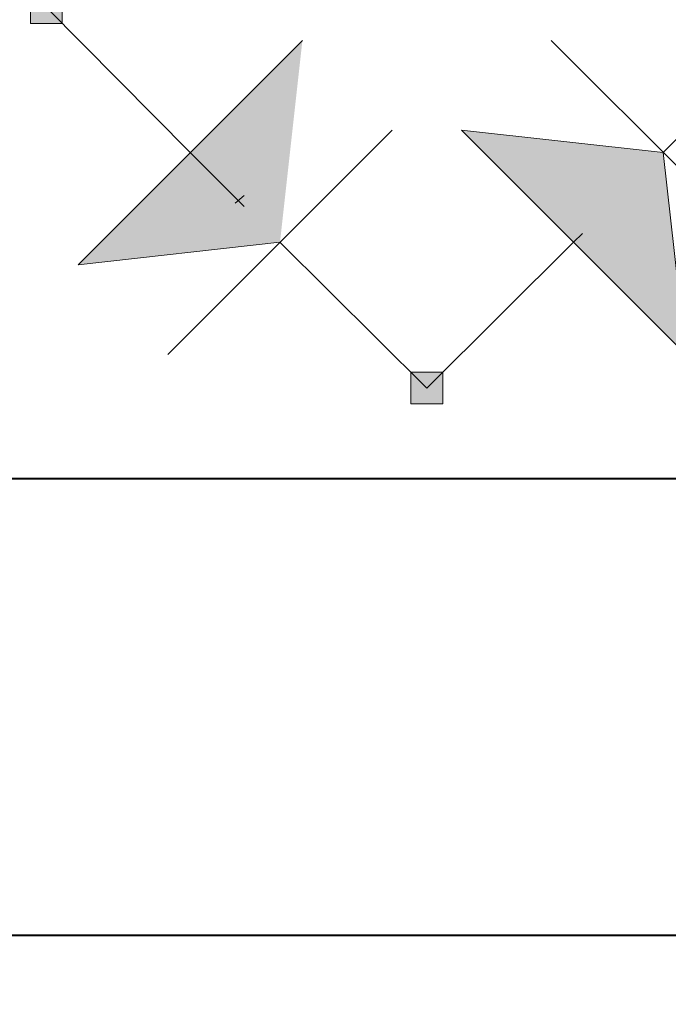
# Model space of a CAD drawing. Units: inches. Extents: x 459864 to 460310, y 324185 to 324787.
# Tile 65 of 112: x 460101.35 to 460114.14, y 324282.12 to 324301.53. Entities that reach past the tile are written whole.
import ezdxf

# ---------------------------------------------------------------- set-up
doc = ezdxf.new("R2010")
doc.units = ezdxf.units.IN
for name, color, linetype, lineweight in [('A-ANNO-DIMS', 2, 'Continuous', 18), ('A-FURN', 8, 'Continuous', 18), ('A-WALL', 7, 'Continuous', 40), ('L-SITE-PATT', 252, 'Continuous', 13)]:
    doc.layers.add(name, color=color, linetype=linetype, lineweight=lineweight)
doc.styles.get("Standard").update_dxf_attribs({"font": 'arial.ttf'})
doc.dimstyles.new('ISO-25', dxfattribs={"dimtxt": 6, "dimasz": 2.5, "dimexe": 1.25, "dimexo": 0.625, "dimtad": 1, "dimdec": 1, "dimlunit": 3, "dimtxsty": 'Standard', "dimcen": 2.5, "dimadec": 0, "dimazin": 0, "dimtfac": 1, "dimtdec": 1, "dimtmove": 0, "dimatfit": 3, "dimfxl": 1, "dimarcsym": 0})

# ---------------------------------------------------------------- blocks, each defined once
blk = doc.blocks.new('Full Wave Bridge')
for p, q in [((0.185922, 0.186729), (0.3, 0.3)), ((0.415786, 0.185084), (0.3, 0.3)), ((0.274311, 0.098341), (0.097534, 0.275118)), ((0.327398, 0.096696), (0.504174, 0.273472)), ((0.504174, 0.273472), (0.486497, 0.114373)), ((0.026823, 0.204407), (0.185922, 0.186729)), ((0.2036, 0.02763), (0.026823, 0.204407)), ((0.398109, 0.025985), (0.574885, 0.202762)), ((0.185922, 0.186729), (0.2036, 0.02763)), ((0.115212, 0.116019), (0.122283, 0.12309)), ((0.115212, 0.116019), (0, 0)), ((0.486497, 0.114373), (0.327398, 0.096696)), ((0.486497, 0.114373), (0.6, 0)), ((0.113504, -0.114373), (0, 0)), ((0.486497, -0.114373), (0.6, 0)), ((0.025116, -0.202762), (0.201892, -0.025985)), ((0.574885, -0.202762), (0.398108, -0.025985)), ((0.095826, -0.273472), (0.272603, -0.096695)), ((0.327398, -0.096695), (0.486497, -0.114373)), ((0.504174, -0.273472), (0.327398, -0.096695)), ((0.113504, -0.114373), (0.120575, -0.121444)), ((0.486497, -0.114373), (0.504174, -0.273472)), ((0.120575, -0.121444), (0.127646, -0.128515)), ((0.127646, -0.128515), (0.134717, -0.135586)), ((0.134717, -0.135586), (0.141788, -0.142657)), ((0.141788, -0.142657), (0.15593, -0.1568)), ((0.155993, -0.148218), (0.148824, -0.154349)), ((0.415786, -0.185084), (0.422857, -0.178013)), ((0.184215, -0.185084), (0.025116, -0.202762)), ((0.184215, -0.185084), (0.3, -0.3)), ((0.415786, -0.185084), (0.3, -0.3))]:
    blk.add_line(p, q)
for points in [[(0.2875, 0.2875), (0.2875, 0.3125), (0.3125, 0.3125), (0.3125, 0.2875)], [(-0.0125, -0.0125), (-0.0125, 0.0125), (0.012501, 0.0125), (0.012501, -0.0125)], [(0.5875, -0.0125), (0.5875, 0.0125), (0.6125, 0.0125), (0.6125, -0.0125)], [(0.2875, -0.3125), (0.2875, -0.2875), (0.3125, -0.2875), (0.3125, -0.3125)]]:
    blk.add_lwpolyline(points, close=True)
for points in [[(0.3125, 0.2875), (0.3125, 0.3125), (0.2875, 0.3125)], [(0.2875, 0.3125), (0.2875, 0.2875), (0.3125, 0.2875)], [(0.327398, 0.096696), (0.486497, 0.114373), (0.504174, 0.273472)], [(0.2036, 0.02763), (0.185922, 0.186729), (0.026823, 0.204407)], [(0.012501, -0.0125), (0.012501, 0.0125), (-0.0125, 0.0125)], [(-0.0125, 0.0125), (-0.0125, -0.0125), (0.012501, -0.0125)], [(0.6125, -0.0125), (0.6125, 0.0125), (0.5875, 0.0125)], [(0.5875, 0.0125), (0.5875, -0.0125), (0.6125, -0.0125)], [(0.025116, -0.202762), (0.184215, -0.185084), (0.201892, -0.025985)], [(0.327398, -0.096695), (0.486497, -0.114373), (0.504174, -0.273472)], [(0.3125, -0.3125), (0.3125, -0.2875), (0.2875, -0.2875)], [(0.2875, -0.2875), (0.2875, -0.3125), (0.3125, -0.3125)]]:
    blk.add_solid(points)
blk = doc.blocks.new('*D73')
at = {"layer": 'A-ANNO-DIMS', "color": 0, "lineweight": -2, "transparency": 16777216}
for p, q in [((460109.617, 324339.904), (460082.316, 324311.465)), ((460063.615, 324291.983), (460080.585, 324309.661))]:
    blk.add_line(p, q, dxfattribs=at)
at = {"layer": 'A-ANNO-DIMS', "color": 0, "transparency": 16777216}
blk.add_solid([(460082.016, 324311.753), (460082.617, 324311.176), (460080.585, 324309.661)], dxfattribs=at)
at = {"layer": 'Defpoints', "color": 0, "transparency": 16777216}
for p in [(460080.585, 324309.661), (460063.615, 324291.983)]:
    blk.add_point(p, dxfattribs=at)
at = {"layer": 'A-ANNO-DIMS', "color": 0, "transparency": 16777216, "insert": (460094.144, 324329.167), "char_height": 6, "attachment_point": 5, "rotation": 46.1701}
blk.add_mtext('R2\'-0 1/2"', dxfattribs=at)

msp = doc.modelspace()

# ---------------------------------------------------------------- hatches: boundary and pattern name
at = {"layer": 'L-SITE-PATT'}
h = msp.add_hatch(dxfattribs=at)
h.set_pattern_fill('DOTS', color=256)
h.paths.add_polyline_path([(460269.804, 324283.483), (460247.115, 324283.483), (460121.929, 324283.483), (460121.929, 324252.473), (460117.429, 324252.473), (460110.124, 324252.473), (460110.124, 324243.287), (460080.83, 324243.287), (460080.83, 324252.473), (460061.115, 324252.473), (460061.115, 324251.882), (460077.909, 324251.882), (460077.909, 324199.483), (460080.83, 324199.483), (460080.83, 324207.553), (460110.124, 324207.553), (460110.124, 324199.483), (460110.813, 324199.483), (460262.115, 324199.483), (460269.804, 324199.483)], flags=17)
edge = h.paths.add_edge_path(flags=0)
edge.add_ellipse((460222.59, 324263.813), major_axis=(-8.485, 8.485), ratio=1, start_angle=405, end_angle=495, ccw=False)
edge.add_line((460214.821, 324254.66), (460214.832, 324254.666))
edge.add_ellipse((460222.59, 324263.813), major_axis=(-8.485, 8.485), ratio=1, start_angle=405, end_angle=495, ccw=False)
edge.add_line((460210.759, 324261.781), (460210.768, 324261.787))
edge.add_ellipse((460222.59, 324263.813), major_axis=(-8.485, 8.485), ratio=1, start_angle=405, end_angle=495, ccw=False)
edge.add_ellipse((460222.59, 324263.813), major_axis=(-8.485, 8.485), ratio=1, start_angle=392.754, end_angle=405, ccw=False)
edge.add_ellipse((460222.59, 324263.813), major_axis=(-8.485, 8.485), ratio=1, start_angle=380.9347, end_angle=392.754, ccw=False)
edge.add_line((460211.337, 324267.985), (460211.34, 324267.985))
edge.add_ellipse((460222.59, 324263.813), major_axis=(-8.485, 8.485), ratio=1, start_angle=380.9347, end_angle=392.754, ccw=False)
edge.add_ellipse((460222.59, 324263.813), major_axis=(-8.485, 8.485), ratio=1, start_angle=347.9015, end_angle=380.9347, ccw=False)
edge.add_ellipse((460222.59, 324263.813), major_axis=(-8.485, 8.485), ratio=1, start_angle=327.0619, end_angle=347.9015, ccw=False)
edge.add_ellipse((460222.59, 324263.813), major_axis=(-8.485, 8.485), ratio=1, start_angle=278.3246, end_angle=327.0619, ccw=False)
edge.add_line((460225.158, 324275.536), (460225.158, 324275.535))
edge.add_ellipse((460222.59, 324263.813), major_axis=(-8.485, 8.485), ratio=1, start_angle=278.3246, end_angle=327.0619, ccw=False)
edge.add_ellipse((460222.59, 324263.813), major_axis=(-8.485, 8.485), ratio=1, start_angle=260.6436, end_angle=278.3246, ccw=False)
edge.add_ellipse((460222.59, 324263.813), major_axis=(-8.485, 8.485), ratio=1, start_angle=225, end_angle=260.6436, ccw=False)
edge.add_line((460234.509, 324265.243), (460234.501, 324265.239))
edge.add_ellipse((460222.59, 324263.813), major_axis=(-8.485, 8.485), ratio=1, start_angle=225, end_angle=260.6436, ccw=False)
edge.add_ellipse((460222.59, 324263.813), major_axis=(-8.485, 8.485), ratio=1, start_angle=495, end_angle=585, ccw=False)
edge.add_line((460234.437, 324261.861), (460234.424, 324261.858))
edge.add_ellipse((460222.59, 324263.813), major_axis=(-8.485, 8.485), ratio=1, start_angle=495, end_angle=585, ccw=False)
edge.add_line((460227.95, 324253.067), (460227.946, 324253.083))
edge.add_ellipse((460222.59, 324263.813), major_axis=(-8.485, 8.485), ratio=1, start_angle=495, end_angle=585, ccw=False)
edge.add_line((460226.223, 324252.369), (460226.211, 324252.38))
edge.add_ellipse((460222.59, 324263.813), major_axis=(-8.485, 8.485), ratio=1, start_angle=495, end_angle=585, ccw=False)
h.paths.add_polyline_path([(460219.651, 324254.347), (460218.461, 324253.545), (460218.275, 324254.789), (460219.642, 324256.542), (460219.625, 324260.848), (460216.11, 324257.333), (460214.35, 324256.978), (460215.416, 324259.356), (460212.524, 324258.496), (460213.137, 324259.93), (460218.507, 324263.813), (460222.59, 324263.813), (460222.59, 324267.807), (460218.176, 324272.212), (460219.026, 324274.639), (460222.59, 324272.811), (460222.59, 324275.423), (460223.057, 324274.825), (460222.675, 324273.492), (460225.912, 324267.135), (460219.625, 324260.848)], flags=0)
edge = h.paths.add_edge_path(flags=0)
edge.add_ellipse((460194.576, 324264.046), major_axis=(-8.485, 8.485), ratio=1, start_angle=495, end_angle=585, ccw=False)
edge.add_line((460199.936, 324253.3), (460199.932, 324253.316))
edge.add_ellipse((460194.576, 324264.046), major_axis=(-8.485, 8.485), ratio=1, start_angle=495, end_angle=585, ccw=False)
edge.add_line((460198.208, 324252.603), (460198.196, 324252.613))
edge.add_ellipse((460194.576, 324264.046), major_axis=(-8.485, 8.485), ratio=1, start_angle=495, end_angle=585, ccw=False)
edge.add_ellipse((460194.576, 324264.046), major_axis=(-8.485, 8.485), ratio=1, start_angle=405, end_angle=495, ccw=False)
edge.add_line((460186.806, 324254.893), (460186.817, 324254.899))
edge.add_ellipse((460194.576, 324264.046), major_axis=(-8.485, 8.485), ratio=1, start_angle=405, end_angle=495, ccw=False)
edge.add_line((460182.744, 324262.014), (460182.753, 324262.02))
edge.add_ellipse((460194.576, 324264.046), major_axis=(-8.485, 8.485), ratio=1, start_angle=405, end_angle=495, ccw=False)
edge.add_ellipse((460194.576, 324264.046), major_axis=(-8.485, 8.485), ratio=1, start_angle=392.754, end_angle=405, ccw=False)
edge.add_ellipse((460194.576, 324264.046), major_axis=(-8.485, 8.485), ratio=1, start_angle=380.9347, end_angle=392.754, ccw=False)
edge.add_line((460183.323, 324268.218), (460183.326, 324268.218))
edge.add_ellipse((460194.576, 324264.046), major_axis=(-8.485, 8.485), ratio=1, start_angle=380.9347, end_angle=392.754, ccw=False)
edge.add_ellipse((460194.576, 324264.046), major_axis=(-8.485, 8.485), ratio=1, start_angle=347.9015, end_angle=380.9347, ccw=False)
edge.add_ellipse((460194.576, 324264.046), major_axis=(-8.485, 8.485), ratio=1, start_angle=327.0619, end_angle=347.9015, ccw=False)
edge.add_ellipse((460194.576, 324264.046), major_axis=(-8.485, 8.485), ratio=1, start_angle=278.3246, end_angle=327.0619, ccw=False)
edge.add_line((460197.144, 324275.769), (460197.143, 324275.768))
edge.add_ellipse((460194.576, 324264.046), major_axis=(-8.485, 8.485), ratio=1, start_angle=278.3246, end_angle=327.0619, ccw=False)
edge.add_ellipse((460194.576, 324264.046), major_axis=(-8.485, 8.485), ratio=1, start_angle=260.6436, end_angle=278.3246, ccw=False)
edge.add_ellipse((460194.576, 324264.046), major_axis=(-8.485, 8.485), ratio=1, start_angle=225, end_angle=260.6436, ccw=False)
edge.add_line((460206.494, 324265.476), (460206.487, 324265.473))
edge.add_ellipse((460194.576, 324264.046), major_axis=(-8.485, 8.485), ratio=1, start_angle=225, end_angle=260.6436, ccw=False)
edge.add_ellipse((460194.576, 324264.046), major_axis=(-8.485, 8.485), ratio=1, start_angle=495, end_angle=585, ccw=False)
edge.add_line((460206.422, 324262.094), (460206.409, 324262.091))
h.paths.add_polyline_path([(460191.61, 324261.081), (460191.637, 324254.58), (460190.447, 324253.778), (460190.261, 324255.023), (460191.628, 324256.775), (460191.61, 324261.081), (460188.096, 324257.566), (460186.335, 324257.211), (460187.402, 324259.589), (460184.509, 324258.729), (460185.123, 324260.163), (460190.493, 324264.046), (460194.576, 324264.046), (460194.576, 324268.04), (460190.161, 324272.446), (460191.011, 324274.872), (460194.576, 324273.044), (460194.576, 324275.657), (460195.043, 324275.058), (460194.661, 324273.725), (460197.897, 324267.368)], flags=0)
edge = h.paths.add_edge_path(flags=0)
edge.add_ellipse((460252.912, 324263.578), major_axis=(-8.485, 8.485), ratio=1, start_angle=405, end_angle=495, ccw=False)
edge.add_line((460241.081, 324261.545), (460241.089, 324261.551))
edge.add_ellipse((460252.912, 324263.578), major_axis=(-8.485, 8.485), ratio=1, start_angle=405, end_angle=495, ccw=False)
edge.add_ellipse((460252.912, 324263.578), major_axis=(-8.485, 8.485), ratio=1, start_angle=392.754, end_angle=405, ccw=False)
edge.add_ellipse((460252.912, 324263.578), major_axis=(-8.485, 8.485), ratio=1, start_angle=380.9347, end_angle=392.754, ccw=False)
edge.add_line((460241.659, 324267.749), (460241.662, 324267.749))
edge.add_ellipse((460252.912, 324263.578), major_axis=(-8.485, 8.485), ratio=1, start_angle=380.9347, end_angle=392.754, ccw=False)
edge.add_ellipse((460252.912, 324263.578), major_axis=(-8.485, 8.485), ratio=1, start_angle=347.9015, end_angle=380.9347, ccw=False)
edge.add_ellipse((460252.912, 324263.578), major_axis=(-8.485, 8.485), ratio=1, start_angle=327.0619, end_angle=347.9015, ccw=False)
edge.add_ellipse((460252.912, 324263.578), major_axis=(-8.485, 8.485), ratio=1, start_angle=278.3246, end_angle=327.0619, ccw=False)
edge.add_line((460255.48, 324275.3), (460255.479, 324275.299))
edge.add_ellipse((460252.912, 324263.578), major_axis=(-8.485, 8.485), ratio=1, start_angle=278.3246, end_angle=327.0619, ccw=False)
edge.add_ellipse((460252.912, 324263.578), major_axis=(-8.485, 8.485), ratio=1, start_angle=260.6436, end_angle=278.3246, ccw=False)
edge.add_ellipse((460252.912, 324263.578), major_axis=(-8.485, 8.485), ratio=1, start_angle=225, end_angle=260.6436, ccw=False)
edge.add_line((460264.83, 324265.007), (460264.823, 324265.004))
edge.add_ellipse((460252.912, 324263.578), major_axis=(-8.485, 8.485), ratio=1, start_angle=225, end_angle=260.6436, ccw=False)
edge.add_ellipse((460252.912, 324263.578), major_axis=(-8.485, 8.485), ratio=1, start_angle=495, end_angle=585, ccw=False)
edge.add_line((460264.758, 324261.626), (460264.745, 324261.622))
edge.add_ellipse((460252.912, 324263.578), major_axis=(-8.485, 8.485), ratio=1, start_angle=495, end_angle=585, ccw=False)
edge.add_line((460258.272, 324252.832), (460258.268, 324252.848))
edge.add_ellipse((460252.912, 324263.578), major_axis=(-8.485, 8.485), ratio=1, start_angle=495, end_angle=585, ccw=False)
edge.add_line((460256.545, 324252.134), (460256.533, 324252.144))
edge.add_ellipse((460252.912, 324263.578), major_axis=(-8.485, 8.485), ratio=1, start_angle=495, end_angle=585, ccw=False)
edge.add_ellipse((460252.912, 324263.578), major_axis=(-8.485, 8.485), ratio=1, start_angle=405, end_angle=495, ccw=False)
edge.add_line((460245.143, 324254.424), (460245.153, 324254.43))
h.paths.add_polyline_path([(460244.672, 324256.742), (460245.738, 324259.12), (460242.846, 324258.26), (460243.459, 324259.694), (460248.829, 324263.578), (460252.912, 324263.578), (460252.912, 324267.571), (460248.497, 324271.977), (460249.348, 324274.403), (460252.912, 324272.576), (460252.912, 324275.188), (460253.379, 324274.589), (460252.997, 324273.257), (460256.233, 324266.899), (460249.946, 324260.612), (460249.973, 324254.111), (460248.783, 324253.309), (460248.597, 324254.554), (460249.964, 324256.306), (460249.946, 324260.612), (460246.432, 324257.097)], flags=0)
edge = h.paths.add_edge_path(flags=0)
edge.add_ellipse((460167.439, 324262.833), major_axis=(-8.485, 8.485), ratio=1, start_angle=495, end_angle=585, ccw=False)
edge.add_line((460172.799, 324252.087), (460172.795, 324252.103))
edge.add_ellipse((460167.439, 324262.833), major_axis=(-8.485, 8.485), ratio=1, start_angle=495, end_angle=585, ccw=False)
edge.add_line((460171.071, 324251.389), (460171.059, 324251.399))
edge.add_ellipse((460167.439, 324262.833), major_axis=(-8.485, 8.485), ratio=1, start_angle=495, end_angle=585, ccw=False)
edge.add_ellipse((460167.439, 324262.833), major_axis=(-8.485, 8.485), ratio=1, start_angle=405, end_angle=495, ccw=False)
edge.add_line((460159.669, 324253.679), (460159.68, 324253.685))
edge.add_ellipse((460167.439, 324262.833), major_axis=(-8.485, 8.485), ratio=1, start_angle=405, end_angle=495, ccw=False)
edge.add_line((460155.607, 324260.8), (460155.616, 324260.806))
edge.add_ellipse((460167.439, 324262.833), major_axis=(-8.485, 8.485), ratio=1, start_angle=405, end_angle=495, ccw=False)
edge.add_ellipse((460167.439, 324262.833), major_axis=(-8.485, 8.485), ratio=1, start_angle=392.754, end_angle=405, ccw=False)
edge.add_ellipse((460167.439, 324262.833), major_axis=(-8.485, 8.485), ratio=1, start_angle=380.9347, end_angle=392.754, ccw=False)
edge.add_line((460156.185, 324267.005), (460156.189, 324267.005))
edge.add_ellipse((460167.439, 324262.833), major_axis=(-8.485, 8.485), ratio=1, start_angle=380.9347, end_angle=392.754, ccw=False)
edge.add_ellipse((460167.439, 324262.833), major_axis=(-8.485, 8.485), ratio=1, start_angle=347.9015, end_angle=380.9347, ccw=False)
edge.add_ellipse((460167.439, 324262.833), major_axis=(-8.485, 8.485), ratio=1, start_angle=327.0619, end_angle=347.9015, ccw=False)
edge.add_ellipse((460167.439, 324262.833), major_axis=(-8.485, 8.485), ratio=1, start_angle=278.3246, end_angle=327.0619, ccw=False)
edge.add_line((460170.007, 324274.556), (460170.006, 324274.554))
edge.add_ellipse((460167.439, 324262.833), major_axis=(-8.485, 8.485), ratio=1, start_angle=278.3246, end_angle=327.0619, ccw=False)
edge.add_ellipse((460167.439, 324262.833), major_axis=(-8.485, 8.485), ratio=1, start_angle=260.6436, end_angle=278.3246, ccw=False)
edge.add_ellipse((460167.439, 324262.833), major_axis=(-8.485, 8.485), ratio=1, start_angle=225, end_angle=260.6436, ccw=False)
edge.add_line((460179.357, 324264.262), (460179.35, 324264.259))
edge.add_ellipse((460167.439, 324262.833), major_axis=(-8.485, 8.485), ratio=1, start_angle=225, end_angle=260.6436, ccw=False)
edge.add_ellipse((460167.439, 324262.833), major_axis=(-8.485, 8.485), ratio=1, start_angle=495, end_angle=585, ccw=False)
edge.add_line((460179.285, 324260.881), (460179.272, 324260.877))
h.paths.add_polyline_path([(460164.473, 324259.867), (460164.5, 324253.366), (460163.31, 324252.565), (460163.124, 324253.809), (460164.491, 324255.561), (460164.473, 324259.867), (460160.958, 324256.353), (460159.198, 324255.998), (460160.265, 324258.375), (460157.372, 324257.515), (460157.986, 324258.949), (460163.356, 324262.833), (460167.439, 324262.833), (460167.439, 324266.826), (460163.024, 324271.232), (460163.874, 324273.659), (460167.439, 324271.831), (460167.439, 324274.443), (460167.905, 324273.844), (460167.524, 324272.512), (460170.76, 324266.154)], flags=0)
edge = h.paths.add_edge_path(flags=0)
edge.add_ellipse((460140.758, 324262.37), major_axis=(-8.485, 8.485), ratio=1, start_angle=495, end_angle=585, ccw=False)
edge.add_line((460146.118, 324251.624), (460146.114, 324251.639))
edge.add_ellipse((460140.758, 324262.37), major_axis=(-8.485, 8.485), ratio=1, start_angle=495, end_angle=585, ccw=False)
edge.add_line((460144.391, 324250.926), (460144.379, 324250.936))
edge.add_ellipse((460140.758, 324262.37), major_axis=(-8.485, 8.485), ratio=1, start_angle=495, end_angle=585, ccw=False)
edge.add_ellipse((460140.758, 324262.37), major_axis=(-8.485, 8.485), ratio=1, start_angle=405, end_angle=495, ccw=False)
edge.add_line((460132.989, 324253.216), (460132.999, 324253.222))
edge.add_ellipse((460140.758, 324262.37), major_axis=(-8.485, 8.485), ratio=1, start_angle=405, end_angle=495, ccw=False)
edge.add_line((460128.927, 324260.337), (460128.935, 324260.343))
edge.add_ellipse((460140.758, 324262.37), major_axis=(-8.485, 8.485), ratio=1, start_angle=405, end_angle=495, ccw=False)
edge.add_ellipse((460140.758, 324262.37), major_axis=(-8.485, 8.485), ratio=1, start_angle=392.754, end_angle=405, ccw=False)
edge.add_ellipse((460140.758, 324262.37), major_axis=(-8.485, 8.485), ratio=1, start_angle=380.9347, end_angle=392.754, ccw=False)
edge.add_line((460129.505, 324266.541), (460129.508, 324266.541))
edge.add_ellipse((460140.758, 324262.37), major_axis=(-8.485, 8.485), ratio=1, start_angle=380.9347, end_angle=392.754, ccw=False)
edge.add_ellipse((460140.758, 324262.37), major_axis=(-8.485, 8.485), ratio=1, start_angle=347.9015, end_angle=380.9347, ccw=False)
edge.add_ellipse((460140.758, 324262.37), major_axis=(-8.485, 8.485), ratio=1, start_angle=327.0619, end_angle=347.9015, ccw=False)
edge.add_ellipse((460140.758, 324262.37), major_axis=(-8.485, 8.485), ratio=1, start_angle=278.3246, end_angle=327.0619, ccw=False)
edge.add_line((460143.326, 324274.092), (460143.325, 324274.091))
edge.add_ellipse((460140.758, 324262.37), major_axis=(-8.485, 8.485), ratio=1, start_angle=278.3246, end_angle=327.0619, ccw=False)
edge.add_ellipse((460140.758, 324262.37), major_axis=(-8.485, 8.485), ratio=1, start_angle=260.6436, end_angle=278.3246, ccw=False)
edge.add_ellipse((460140.758, 324262.37), major_axis=(-8.485, 8.485), ratio=1, start_angle=225, end_angle=260.6436, ccw=False)
edge.add_line((460152.677, 324263.799), (460152.669, 324263.796))
edge.add_ellipse((460140.758, 324262.37), major_axis=(-8.485, 8.485), ratio=1, start_angle=225, end_angle=260.6436, ccw=False)
edge.add_ellipse((460140.758, 324262.37), major_axis=(-8.485, 8.485), ratio=1, start_angle=495, end_angle=585, ccw=False)
edge.add_line((460152.604, 324260.418), (460152.592, 324260.414))
h.paths.add_polyline_path([(460137.792, 324259.404), (460137.819, 324252.903), (460136.629, 324252.101), (460136.443, 324253.346), (460137.81, 324255.098), (460137.792, 324259.404), (460134.278, 324255.889), (460132.518, 324255.534), (460133.584, 324257.912), (460130.692, 324257.052), (460131.305, 324258.486), (460136.675, 324262.37), (460140.758, 324262.37), (460140.758, 324266.363), (460136.343, 324270.769), (460137.194, 324273.195), (460140.758, 324271.367), (460140.758, 324273.98), (460141.225, 324273.381), (460140.843, 324272.049), (460144.079, 324265.691)], flags=0)
h.paths.add_polyline_path([(460110.124, 324227.414), (460080.83, 324227.414), (460080.83, 324235.484), (460110.124, 324235.484)], flags=16)
h.paths.add_polyline_path([(460110.124, 324220.797), (460110.124, 324212.727), (460080.83, 324212.727), (460080.83, 324220.797)], flags=16)
h.paths.add_polyline_path([(460269.804, 324283.483), (460247.115, 324283.483), (460121.929, 324283.483), (460121.929, 324252.473), (460117.429, 324252.473), (460110.124, 324252.473), (460110.124, 324243.287), (460080.83, 324243.287), (460080.83, 324252.473), (460061.115, 324252.473), (460061.115, 324251.882), (460077.909, 324251.882), (460077.909, 324199.483), (460080.83, 324199.483), (460080.83, 324207.553), (460110.124, 324207.553), (460110.124, 324199.483), (460262.115, 324199.483), (460269.804, 324199.483)], flags=17)
h.paths.add_polyline_path([(460219.651, 324254.347), (460218.461, 324253.545), (460218.275, 324254.789), (460219.642, 324256.542), (460219.625, 324260.848), (460216.11, 324257.333), (460214.35, 324256.978), (460215.416, 324259.356), (460212.524, 324258.496), (460213.137, 324259.93), (460218.507, 324263.813), (460222.59, 324263.813), (460220.18, 324266.223), (460215.461, 324265.308), (460211.835, 324266.137), (460216.247, 324267.985), (460218.418, 324267.985), (460222.59, 324263.813), (460222.59, 324267.807), (460218.176, 324272.212), (460219.026, 324274.639), (460222.59, 324272.811), (460222.59, 324275.423), (460223.057, 324274.825), (460222.675, 324273.492), (460225.912, 324267.135), (460222.59, 324263.813), (460231.383, 324263.813), (460228.485, 324262.488), (460224.425, 324261.978), (460228.68, 324257.724), (460228.966, 324254.791), (460227.142, 324256.537), (460227.542, 324254.819), (460227.333, 324253.614), (460222.59, 324259.985), (460222.59, 324255.497), (460221.377, 324256.541), (460220.576, 324261.799), (460219.625, 324260.848)], flags=0)
h.paths.add_polyline_path([(460199.127, 324256.77), (460199.528, 324255.052), (460199.319, 324253.848), (460194.576, 324260.218), (460194.576, 324255.73), (460193.363, 324256.774), (460192.561, 324262.032), (460191.61, 324261.081), (460191.637, 324254.58), (460190.447, 324253.778), (460190.261, 324255.023), (460191.628, 324256.775), (460191.61, 324261.081), (460188.096, 324257.566), (460186.335, 324257.211), (460187.402, 324259.589), (460184.509, 324258.729), (460185.123, 324260.163), (460190.493, 324264.046), (460194.576, 324264.046), (460192.166, 324266.456), (460187.446, 324265.541), (460183.82, 324266.37), (460188.232, 324268.218), (460190.404, 324268.218), (460194.576, 324264.046), (460194.576, 324268.04), (460190.161, 324272.446), (460191.011, 324274.872), (460194.576, 324273.044), (460194.576, 324275.657), (460195.043, 324275.058), (460194.661, 324273.725), (460197.897, 324267.368), (460194.576, 324264.046), (460203.368, 324264.046), (460200.47, 324262.721), (460196.411, 324262.212), (460200.665, 324257.957), (460200.951, 324255.024)], flags=0)
h.paths.add_polyline_path([(460244.672, 324256.742), (460245.738, 324259.12), (460242.846, 324258.26), (460243.459, 324259.694), (460248.829, 324263.578), (460252.912, 324263.578), (460250.502, 324265.987), (460245.783, 324265.072), (460242.156, 324265.901), (460246.568, 324267.749), (460248.74, 324267.749), (460252.912, 324263.578), (460252.912, 324267.571), (460248.497, 324271.977), (460249.348, 324274.403), (460252.912, 324272.576), (460252.912, 324275.188), (460253.379, 324274.589), (460252.997, 324273.257), (460256.233, 324266.899), (460252.912, 324263.578), (460261.705, 324263.578), (460258.806, 324262.252), (460254.747, 324261.743), (460259.002, 324257.488), (460259.288, 324254.555), (460257.463, 324256.301), (460257.864, 324254.583), (460257.655, 324253.379), (460252.912, 324259.749), (460252.912, 324255.261), (460251.699, 324256.305), (460250.897, 324261.563), (460249.946, 324260.612), (460249.973, 324254.111), (460248.783, 324253.309), (460248.597, 324254.554), (460249.964, 324256.306), (460249.946, 324260.612), (460246.432, 324257.097)], flags=0)
h.paths.add_polyline_path([(460173.528, 324256.743), (460173.814, 324253.811), (460171.99, 324255.556), (460172.39, 324253.838), (460172.182, 324252.634), (460167.439, 324259.004), (460167.439, 324254.516), (460166.226, 324255.56), (460165.424, 324260.818), (460164.473, 324259.867), (460164.5, 324253.366), (460163.31, 324252.565), (460163.124, 324253.809), (460164.491, 324255.561), (460164.473, 324259.867), (460160.958, 324256.353), (460159.198, 324255.998), (460160.265, 324258.375), (460157.372, 324257.515), (460157.986, 324258.949), (460163.356, 324262.833), (460167.439, 324262.833), (460165.029, 324265.243), (460160.309, 324264.327), (460156.683, 324265.156), (460161.095, 324267.005), (460163.267, 324267.005), (460167.439, 324262.833), (460167.439, 324266.826), (460163.024, 324271.232), (460163.874, 324273.659), (460167.439, 324271.831), (460167.439, 324274.443), (460167.905, 324273.844), (460167.524, 324272.512), (460170.76, 324266.154), (460167.439, 324262.833), (460176.231, 324262.833), (460173.333, 324261.507), (460169.274, 324260.998)], flags=0)
h.paths.add_polyline_path([(460146.848, 324256.28), (460147.134, 324253.347), (460145.31, 324255.093), (460145.71, 324253.375), (460145.501, 324252.171), (460140.758, 324258.541), (460140.758, 324254.053), (460139.545, 324255.097), (460138.744, 324260.355), (460137.792, 324259.404), (460137.819, 324252.903), (460136.629, 324252.101), (460136.443, 324253.346), (460137.81, 324255.098), (460137.792, 324259.404), (460134.278, 324255.889), (460132.518, 324255.534), (460133.584, 324257.912), (460130.692, 324257.052), (460131.305, 324258.486), (460136.675, 324262.37), (460140.758, 324262.37), (460138.348, 324264.779), (460133.629, 324263.864), (460130.002, 324264.693), (460134.414, 324266.541), (460136.586, 324266.541), (460140.758, 324262.37), (460140.758, 324266.363), (460136.343, 324270.769), (460137.194, 324273.195), (460140.758, 324271.367), (460140.758, 324273.98), (460141.225, 324273.381), (460140.843, 324272.049), (460144.079, 324265.691), (460140.758, 324262.37), (460149.551, 324262.37), (460146.653, 324261.044), (460142.593, 324260.535)], flags=0)
edge = h.paths.add_edge_path()
edge.add_line((460269.804, 324272.549), (460260.881, 324272.549))
edge.add_ellipse((460252.912, 324263.578), major_axis=(-8.485, 8.485), ratio=1, start_angle=260.6436, end_angle=273.3846, ccw=False)
edge.add_line((460262.283, 324271.092), (460262.261, 324271.091))
edge.add_ellipse((460252.912, 324263.578), major_axis=(-8.485, 8.485), ratio=1, start_angle=260.6436, end_angle=273.3846, ccw=False)
edge.add_ellipse((460252.912, 324263.578), major_axis=(-8.485, 8.485), ratio=1, start_angle=225, end_angle=260.6436, ccw=False)
edge.add_line((460263.609, 324269.063), (460263.572, 324269.058))
edge.add_ellipse((460252.912, 324263.578), major_axis=(-8.485, 8.485), ratio=1, start_angle=225, end_angle=260.6436, ccw=False)
edge.add_line((460264.615, 324266.306), (460264.585, 324266.305))
edge.add_ellipse((460252.912, 324263.578), major_axis=(-8.485, 8.485), ratio=1, start_angle=225, end_angle=260.6436, ccw=False)
edge.add_line((460264.83, 324265.007), (460264.823, 324265.004))
edge.add_ellipse((460252.912, 324263.578), major_axis=(-8.485, 8.485), ratio=1, start_angle=225, end_angle=260.6436, ccw=False)
edge.add_ellipse((460252.912, 324263.578), major_axis=(-8.485, 8.485), ratio=1, start_angle=495, end_angle=585, ccw=False)
edge.add_line((460264.758, 324261.626), (460264.745, 324261.622))
edge.add_ellipse((460252.912, 324263.578), major_axis=(-8.485, 8.485), ratio=1, start_angle=495, end_angle=585, ccw=False)
edge.add_line((460263.442, 324257.739), (460263.389, 324257.779))
edge.add_ellipse((460252.912, 324263.578), major_axis=(-8.485, 8.485), ratio=1, start_angle=495, end_angle=585, ccw=False)
edge.add_line((460258.128, 324252.744), (460258.102, 324252.779))
edge.add_ellipse((460252.912, 324263.578), major_axis=(-8.485, 8.485), ratio=1, start_angle=495, end_angle=585, ccw=False)
edge.add_line((460256.545, 324252.134), (460256.533, 324252.144))
edge.add_ellipse((460252.912, 324263.578), major_axis=(-8.485, 8.485), ratio=1, start_angle=495, end_angle=585, ccw=False)
edge.add_ellipse((460252.912, 324263.578), major_axis=(-8.485, 8.485), ratio=1, start_angle=405, end_angle=495, ccw=False)
edge.add_line((460250.594, 324251.78), (460250.605, 324251.82))
edge.add_ellipse((460252.912, 324263.578), major_axis=(-8.485, 8.485), ratio=1, start_angle=405, end_angle=495, ccw=False)
edge.add_line((460245.143, 324254.424), (460245.153, 324254.43))
edge.add_ellipse((460252.912, 324263.578), major_axis=(-8.485, 8.485), ratio=1, start_angle=405, end_angle=495, ccw=False)
edge.add_line((460243.525, 324256.059), (460243.56, 324256.091))
edge.add_ellipse((460252.912, 324263.578), major_axis=(-8.485, 8.485), ratio=1, start_angle=405, end_angle=495, ccw=False)
edge.add_line((460241.44, 324259.893), (460241.522, 324259.896))
edge.add_ellipse((460252.912, 324263.578), major_axis=(-8.485, 8.485), ratio=1, start_angle=405, end_angle=495, ccw=False)
edge.add_line((460241.081, 324261.545), (460241.089, 324261.551))
edge.add_ellipse((460252.912, 324263.578), major_axis=(-8.485, 8.485), ratio=1, start_angle=405, end_angle=495, ccw=False)
edge.add_ellipse((460252.912, 324263.578), major_axis=(-8.485, 8.485), ratio=1, start_angle=392.754, end_angle=405, ccw=False)
edge.add_line((460241.05, 324265.438), (460241.063, 324265.443))
edge.add_ellipse((460252.912, 324263.578), major_axis=(-8.485, 8.485), ratio=1, start_angle=392.754, end_angle=405, ccw=False)
edge.add_ellipse((460252.912, 324263.578), major_axis=(-8.485, 8.485), ratio=1, start_angle=380.9347, end_angle=392.754, ccw=False)
edge.add_line((460241.452, 324267.176), (460241.469, 324267.171))
edge.add_ellipse((460252.912, 324263.578), major_axis=(-8.485, 8.485), ratio=1, start_angle=380.9347, end_angle=392.754, ccw=False)
edge.add_line((460241.659, 324267.749), (460241.662, 324267.749))
edge.add_ellipse((460252.912, 324263.578), major_axis=(-8.485, 8.485), ratio=1, start_angle=380.9347, end_angle=392.754, ccw=False)
edge.add_ellipse((460252.912, 324263.578), major_axis=(-8.485, 8.485), ratio=1, start_angle=356.6154, end_angle=380.9347, ccw=False)
edge.add_line((460244.88, 324272.488), (460244.713, 324272.549))
edge.add_line((460244.713, 324272.549), (460230.817, 324272.549))
edge.add_ellipse((460222.59, 324263.813), major_axis=(-8.485, 8.485), ratio=1, start_angle=260.6436, end_angle=271.7178, ccw=False)
edge.add_ellipse((460222.59, 324263.813), major_axis=(-8.485, 8.485), ratio=1, start_angle=225, end_angle=260.6436, ccw=False)
edge.add_line((460233.287, 324269.299), (460233.25, 324269.294))
edge.add_ellipse((460222.59, 324263.813), major_axis=(-8.485, 8.485), ratio=1, start_angle=225, end_angle=260.6436, ccw=False)
edge.add_line((460234.294, 324266.541), (460234.264, 324266.541))
edge.add_ellipse((460222.59, 324263.813), major_axis=(-8.485, 8.485), ratio=1, start_angle=225, end_angle=260.6436, ccw=False)
edge.add_line((460234.509, 324265.243), (460234.501, 324265.239))
edge.add_ellipse((460222.59, 324263.813), major_axis=(-8.485, 8.485), ratio=1, start_angle=225, end_angle=260.6436, ccw=False)
edge.add_ellipse((460222.59, 324263.813), major_axis=(-8.485, 8.485), ratio=1, start_angle=495, end_angle=585, ccw=False)
edge.add_line((460234.437, 324261.861), (460234.424, 324261.858))
edge.add_ellipse((460222.59, 324263.813), major_axis=(-8.485, 8.485), ratio=1, start_angle=495, end_angle=585, ccw=False)
edge.add_line((460233.121, 324257.975), (460233.068, 324258.015))
edge.add_ellipse((460222.59, 324263.813), major_axis=(-8.485, 8.485), ratio=1, start_angle=495, end_angle=585, ccw=False)
edge.add_line((460227.806, 324252.979), (460227.78, 324253.014))
edge.add_ellipse((460222.59, 324263.813), major_axis=(-8.485, 8.485), ratio=1, start_angle=495, end_angle=585, ccw=False)
edge.add_line((460226.223, 324252.369), (460226.211, 324252.38))
edge.add_ellipse((460222.59, 324263.813), major_axis=(-8.485, 8.485), ratio=1, start_angle=495, end_angle=585, ccw=False)
edge.add_ellipse((460222.59, 324263.813), major_axis=(-8.485, 8.485), ratio=1, start_angle=405, end_angle=495, ccw=False)
edge.add_line((460220.272, 324252.016), (460220.283, 324252.055))
edge.add_ellipse((460222.59, 324263.813), major_axis=(-8.485, 8.485), ratio=1, start_angle=405, end_angle=495, ccw=False)
edge.add_line((460214.821, 324254.66), (460214.832, 324254.666))
edge.add_ellipse((460222.59, 324263.813), major_axis=(-8.485, 8.485), ratio=1, start_angle=405, end_angle=495, ccw=False)
edge.add_line((460213.203, 324256.295), (460213.239, 324256.327))
edge.add_ellipse((460222.59, 324263.813), major_axis=(-8.485, 8.485), ratio=1, start_angle=405, end_angle=495, ccw=False)
edge.add_line((460211.118, 324260.128), (460211.201, 324260.131))
edge.add_ellipse((460222.59, 324263.813), major_axis=(-8.485, 8.485), ratio=1, start_angle=405, end_angle=495, ccw=False)
edge.add_line((460210.759, 324261.781), (460210.768, 324261.787))
edge.add_ellipse((460222.59, 324263.813), major_axis=(-8.485, 8.485), ratio=1, start_angle=405, end_angle=495, ccw=False)
edge.add_ellipse((460222.59, 324263.813), major_axis=(-8.485, 8.485), ratio=1, start_angle=392.754, end_angle=405, ccw=False)
edge.add_line((460210.729, 324265.673), (460210.741, 324265.678))
edge.add_ellipse((460222.59, 324263.813), major_axis=(-8.485, 8.485), ratio=1, start_angle=392.754, end_angle=405, ccw=False)
edge.add_ellipse((460222.59, 324263.813), major_axis=(-8.485, 8.485), ratio=1, start_angle=380.9347, end_angle=392.754, ccw=False)
edge.add_line((460211.13, 324267.412), (460211.147, 324267.407))
edge.add_ellipse((460222.59, 324263.813), major_axis=(-8.485, 8.485), ratio=1, start_angle=380.9347, end_angle=392.754, ccw=False)
edge.add_line((460211.337, 324267.985), (460211.34, 324267.985))
edge.add_ellipse((460222.59, 324263.813), major_axis=(-8.485, 8.485), ratio=1, start_angle=380.9347, end_angle=392.754, ccw=False)
edge.add_ellipse((460222.59, 324263.813), major_axis=(-8.485, 8.485), ratio=1, start_angle=358.2822, end_angle=380.9347, ccw=False)
edge.add_line((460213.705, 324271.902), (460213.709, 324271.869))
edge.add_ellipse((460222.59, 324263.813), major_axis=(-8.485, 8.485), ratio=1, start_angle=358.2822, end_angle=380.9347, ccw=False)
edge.add_line((460214.363, 324272.549), (460203.078, 324272.549))
edge.add_line((460203.078, 324272.549), (460203.06, 324272.531))
edge.add_ellipse((460194.576, 324264.046), major_axis=(-8.485, 8.485), ratio=1, start_angle=260.6436, end_angle=270.1168, ccw=False)
edge.add_line((460203.957, 324271.561), (460203.921, 324271.56))
edge.add_ellipse((460194.576, 324264.046), major_axis=(-8.485, 8.485), ratio=1, start_angle=260.6436, end_angle=270.1168, ccw=False)
edge.add_ellipse((460194.576, 324264.046), major_axis=(-8.485, 8.485), ratio=1, start_angle=225, end_angle=260.6436, ccw=False)
edge.add_line((460205.272, 324269.532), (460205.235, 324269.527))
edge.add_ellipse((460194.576, 324264.046), major_axis=(-8.485, 8.485), ratio=1, start_angle=225, end_angle=260.6436, ccw=False)
edge.add_line((460206.279, 324266.774), (460206.249, 324266.774))
edge.add_ellipse((460194.576, 324264.046), major_axis=(-8.485, 8.485), ratio=1, start_angle=225, end_angle=260.6436, ccw=False)
edge.add_line((460206.494, 324265.476), (460206.487, 324265.473))
edge.add_ellipse((460194.576, 324264.046), major_axis=(-8.485, 8.485), ratio=1, start_angle=225, end_angle=260.6436, ccw=False)
edge.add_ellipse((460194.576, 324264.046), major_axis=(-8.485, 8.485), ratio=1, start_angle=495, end_angle=585, ccw=False)
edge.add_line((460206.422, 324262.094), (460206.409, 324262.091))
edge.add_ellipse((460194.576, 324264.046), major_axis=(-8.485, 8.485), ratio=1, start_angle=495, end_angle=585, ccw=False)
edge.add_line((460205.106, 324258.208), (460205.053, 324258.248))
edge.add_ellipse((460194.576, 324264.046), major_axis=(-8.485, 8.485), ratio=1, start_angle=495, end_angle=585, ccw=False)
edge.add_line((460199.792, 324253.212), (460199.766, 324253.248))
edge.add_ellipse((460194.576, 324264.046), major_axis=(-8.485, 8.485), ratio=1, start_angle=495, end_angle=585, ccw=False)
edge.add_line((460198.208, 324252.603), (460198.196, 324252.613))
edge.add_ellipse((460194.576, 324264.046), major_axis=(-8.485, 8.485), ratio=1, start_angle=495, end_angle=585, ccw=False)
edge.add_ellipse((460194.576, 324264.046), major_axis=(-8.485, 8.485), ratio=1, start_angle=405, end_angle=495, ccw=False)
edge.add_line((460192.258, 324252.249), (460192.268, 324252.289))
edge.add_ellipse((460194.576, 324264.046), major_axis=(-8.485, 8.485), ratio=1, start_angle=405, end_angle=495, ccw=False)
edge.add_line((460186.806, 324254.893), (460186.817, 324254.899))
edge.add_ellipse((460194.576, 324264.046), major_axis=(-8.485, 8.485), ratio=1, start_angle=405, end_angle=495, ccw=False)
edge.add_line((460185.188, 324256.528), (460185.224, 324256.56))
edge.add_ellipse((460194.576, 324264.046), major_axis=(-8.485, 8.485), ratio=1, start_angle=405, end_angle=495, ccw=False)
edge.add_line((460183.104, 324260.362), (460183.186, 324260.365))
edge.add_ellipse((460194.576, 324264.046), major_axis=(-8.485, 8.485), ratio=1, start_angle=405, end_angle=495, ccw=False)
edge.add_line((460182.744, 324262.014), (460182.753, 324262.02))
edge.add_ellipse((460194.576, 324264.046), major_axis=(-8.485, 8.485), ratio=1, start_angle=405, end_angle=495, ccw=False)
edge.add_ellipse((460194.576, 324264.046), major_axis=(-8.485, 8.485), ratio=1, start_angle=392.754, end_angle=405, ccw=False)
edge.add_line((460182.714, 324265.906), (460182.726, 324265.912))
edge.add_ellipse((460194.576, 324264.046), major_axis=(-8.485, 8.485), ratio=1, start_angle=392.754, end_angle=405, ccw=False)
edge.add_ellipse((460194.576, 324264.046), major_axis=(-8.485, 8.485), ratio=1, start_angle=380.9347, end_angle=392.754, ccw=False)
edge.add_line((460183.116, 324267.645), (460183.133, 324267.64))
edge.add_ellipse((460194.576, 324264.046), major_axis=(-8.485, 8.485), ratio=1, start_angle=380.9347, end_angle=392.754, ccw=False)
edge.add_line((460183.323, 324268.218), (460183.326, 324268.218))
edge.add_ellipse((460194.576, 324264.046), major_axis=(-8.485, 8.485), ratio=1, start_angle=380.9347, end_angle=392.754, ccw=False)
edge.add_ellipse((460194.576, 324264.046), major_axis=(-8.485, 8.485), ratio=1, start_angle=359.8832, end_angle=380.9347, ccw=False)
edge.add_line((460184.491, 324270.611), (460184.553, 324270.611))
edge.add_ellipse((460194.576, 324264.046), major_axis=(-8.485, 8.485), ratio=1, start_angle=359.8832, end_angle=380.9347, ccw=False)
edge.add_line((460185.346, 324271.76), (460185.379, 324271.728))
edge.add_ellipse((460194.576, 324264.046), major_axis=(-8.485, 8.485), ratio=1, start_angle=359.8832, end_angle=380.9347, ccw=False)
edge.add_line((460185.697, 324272.086), (460185.633, 324272.549))
edge.add_line((460185.633, 324272.549), (460174.683, 324272.549))
edge.add_line((460174.683, 324272.549), (460174.606, 324272.457))
edge.add_ellipse((460167.439, 324262.833), major_axis=(-8.485, 8.485), ratio=1, start_angle=260.6436, end_angle=278.3246, ccw=False)
edge.add_ellipse((460167.439, 324262.833), major_axis=(-8.485, 8.485), ratio=1, start_angle=225, end_angle=260.6436, ccw=False)
edge.add_line((460178.135, 324268.318), (460178.098, 324268.313))
edge.add_ellipse((460167.439, 324262.833), major_axis=(-8.485, 8.485), ratio=1, start_angle=225, end_angle=260.6436, ccw=False)
edge.add_line((460179.142, 324265.561), (460179.112, 324265.56))
edge.add_ellipse((460167.439, 324262.833), major_axis=(-8.485, 8.485), ratio=1, start_angle=225, end_angle=260.6436, ccw=False)
edge.add_line((460179.357, 324264.262), (460179.35, 324264.259))
edge.add_ellipse((460167.439, 324262.833), major_axis=(-8.485, 8.485), ratio=1, start_angle=225, end_angle=260.6436, ccw=False)
edge.add_ellipse((460167.439, 324262.833), major_axis=(-8.485, 8.485), ratio=1, start_angle=495, end_angle=585, ccw=False)
edge.add_line((460179.285, 324260.881), (460179.272, 324260.877))
edge.add_ellipse((460167.439, 324262.833), major_axis=(-8.485, 8.485), ratio=1, start_angle=495, end_angle=585, ccw=False)
edge.add_line((460177.969, 324256.994), (460177.916, 324257.034))
edge.add_ellipse((460167.439, 324262.833), major_axis=(-8.485, 8.485), ratio=1, start_angle=495, end_angle=585, ccw=False)
edge.add_line((460172.655, 324251.999), (460172.629, 324252.034))
edge.add_ellipse((460167.439, 324262.833), major_axis=(-8.485, 8.485), ratio=1, start_angle=495, end_angle=585, ccw=False)
edge.add_line((460171.071, 324251.389), (460171.059, 324251.399))
edge.add_ellipse((460167.439, 324262.833), major_axis=(-8.485, 8.485), ratio=1, start_angle=495, end_angle=585, ccw=False)
edge.add_ellipse((460167.439, 324262.833), major_axis=(-8.485, 8.485), ratio=1, start_angle=405, end_angle=495, ccw=False)
edge.add_line((460165.121, 324251.036), (460165.131, 324251.075))
edge.add_ellipse((460167.439, 324262.833), major_axis=(-8.485, 8.485), ratio=1, start_angle=405, end_angle=495, ccw=False)
edge.add_line((460159.669, 324253.679), (460159.68, 324253.685))
edge.add_ellipse((460167.439, 324262.833), major_axis=(-8.485, 8.485), ratio=1, start_angle=405, end_angle=495, ccw=False)
edge.add_line((460158.051, 324255.314), (460158.087, 324255.347))
edge.add_ellipse((460167.439, 324262.833), major_axis=(-8.485, 8.485), ratio=1, start_angle=405, end_angle=495, ccw=False)
edge.add_line((460155.967, 324259.148), (460156.049, 324259.151))
edge.add_ellipse((460167.439, 324262.833), major_axis=(-8.485, 8.485), ratio=1, start_angle=405, end_angle=495, ccw=False)
edge.add_line((460155.607, 324260.8), (460155.616, 324260.806))
edge.add_ellipse((460167.439, 324262.833), major_axis=(-8.485, 8.485), ratio=1, start_angle=405, end_angle=495, ccw=False)
edge.add_ellipse((460167.439, 324262.833), major_axis=(-8.485, 8.485), ratio=1, start_angle=392.754, end_angle=405, ccw=False)
edge.add_line((460155.577, 324264.693), (460155.589, 324264.698))
edge.add_ellipse((460167.439, 324262.833), major_axis=(-8.485, 8.485), ratio=1, start_angle=392.754, end_angle=405, ccw=False)
edge.add_ellipse((460167.439, 324262.833), major_axis=(-8.485, 8.485), ratio=1, start_angle=380.9347, end_angle=392.754, ccw=False)
edge.add_line((460155.979, 324266.432), (460155.996, 324266.426))
edge.add_ellipse((460167.439, 324262.833), major_axis=(-8.485, 8.485), ratio=1, start_angle=380.9347, end_angle=392.754, ccw=False)
edge.add_line((460156.185, 324267.005), (460156.189, 324267.005))
edge.add_ellipse((460167.439, 324262.833), major_axis=(-8.485, 8.485), ratio=1, start_angle=380.9347, end_angle=392.754, ccw=False)
edge.add_ellipse((460167.439, 324262.833), major_axis=(-8.485, 8.485), ratio=1, start_angle=350.9345, end_angle=380.9347, ccw=False)
edge.add_line((460157.363, 324269.397), (460157.414, 324269.397))
edge.add_ellipse((460167.439, 324262.833), major_axis=(-8.485, 8.485), ratio=1, start_angle=350.9345, end_angle=380.9347, ccw=False)
edge.add_line((460158.221, 324270.535), (460158.236, 324270.519))
edge.add_ellipse((460167.439, 324262.833), major_axis=(-8.485, 8.485), ratio=1, start_angle=350.9345, end_angle=380.9347, ccw=False)
edge.add_line((460159.379, 324271.753), (460159.419, 324271.738))
edge.add_ellipse((460167.439, 324262.833), major_axis=(-8.485, 8.485), ratio=1, start_angle=350.9345, end_angle=380.9347, ccw=False)
edge.add_line((460160.396, 324272.549), (460147.112, 324272.549))
edge.add_ellipse((460140.758, 324262.37), major_axis=(-8.485, 8.485), ratio=1, start_angle=278.3246, end_angle=283.0261, ccw=False)
edge.add_ellipse((460140.758, 324262.37), major_axis=(-8.485, 8.485), ratio=1, start_angle=260.6436, end_angle=278.3246, ccw=False)
edge.add_ellipse((460140.758, 324262.37), major_axis=(-8.485, 8.485), ratio=1, start_angle=225, end_angle=260.6436, ccw=False)
edge.add_line((460151.455, 324267.855), (460151.418, 324267.85))
edge.add_ellipse((460140.758, 324262.37), major_axis=(-8.485, 8.485), ratio=1, start_angle=225, end_angle=260.6436, ccw=False)
edge.add_line((460152.462, 324265.098), (460152.431, 324265.097))
edge.add_ellipse((460140.758, 324262.37), major_axis=(-8.485, 8.485), ratio=1, start_angle=225, end_angle=260.6436, ccw=False)
edge.add_line((460152.677, 324263.799), (460152.669, 324263.796))
edge.add_ellipse((460140.758, 324262.37), major_axis=(-8.485, 8.485), ratio=1, start_angle=225, end_angle=260.6436, ccw=False)
edge.add_ellipse((460140.758, 324262.37), major_axis=(-8.485, 8.485), ratio=1, start_angle=495, end_angle=585, ccw=False)
edge.add_line((460152.604, 324260.418), (460152.592, 324260.414))
edge.add_ellipse((460140.758, 324262.37), major_axis=(-8.485, 8.485), ratio=1, start_angle=495, end_angle=585, ccw=False)
edge.add_line((460151.288, 324256.531), (460151.235, 324256.571))
edge.add_ellipse((460140.758, 324262.37), major_axis=(-8.485, 8.485), ratio=1, start_angle=495, end_angle=585, ccw=False)
edge.add_line((460145.974, 324251.535), (460145.948, 324251.571))
edge.add_ellipse((460140.758, 324262.37), major_axis=(-8.485, 8.485), ratio=1, start_angle=495, end_angle=585, ccw=False)
edge.add_line((460144.391, 324250.926), (460144.379, 324250.936))
edge.add_ellipse((460140.758, 324262.37), major_axis=(-8.485, 8.485), ratio=1, start_angle=495, end_angle=585, ccw=False)
edge.add_ellipse((460140.758, 324262.37), major_axis=(-8.485, 8.485), ratio=1, start_angle=405, end_angle=495, ccw=False)
edge.add_line((460138.44, 324250.572), (460138.451, 324250.612))
edge.add_ellipse((460140.758, 324262.37), major_axis=(-8.485, 8.485), ratio=1, start_angle=405, end_angle=495, ccw=False)
edge.add_line((460132.989, 324253.216), (460132.999, 324253.222))
edge.add_ellipse((460140.758, 324262.37), major_axis=(-8.485, 8.485), ratio=1, start_angle=405, end_angle=495, ccw=False)
edge.add_line((460131.371, 324254.851), (460131.406, 324254.883))
edge.add_ellipse((460140.758, 324262.37), major_axis=(-8.485, 8.485), ratio=1, start_angle=405, end_angle=495, ccw=False)
edge.add_line((460129.286, 324258.685), (460129.369, 324258.688))
edge.add_ellipse((460140.758, 324262.37), major_axis=(-8.485, 8.485), ratio=1, start_angle=405, end_angle=495, ccw=False)
edge.add_line((460128.927, 324260.337), (460128.935, 324260.343))
edge.add_ellipse((460140.758, 324262.37), major_axis=(-8.485, 8.485), ratio=1, start_angle=405, end_angle=495, ccw=False)
edge.add_ellipse((460140.758, 324262.37), major_axis=(-8.485, 8.485), ratio=1, start_angle=392.754, end_angle=405, ccw=False)
edge.add_line((460128.896, 324264.23), (460128.909, 324264.235))
edge.add_ellipse((460140.758, 324262.37), major_axis=(-8.485, 8.485), ratio=1, start_angle=392.754, end_angle=405, ccw=False)
edge.add_ellipse((460140.758, 324262.37), major_axis=(-8.485, 8.485), ratio=1, start_angle=380.9347, end_angle=392.754, ccw=False)
edge.add_line((460129.298, 324265.968), (460129.315, 324265.963))
edge.add_ellipse((460140.758, 324262.37), major_axis=(-8.485, 8.485), ratio=1, start_angle=380.9347, end_angle=392.754, ccw=False)
edge.add_line((460129.505, 324266.541), (460129.508, 324266.541))
edge.add_ellipse((460140.758, 324262.37), major_axis=(-8.485, 8.485), ratio=1, start_angle=380.9347, end_angle=392.754, ccw=False)
edge.add_ellipse((460140.758, 324262.37), major_axis=(-8.485, 8.485), ratio=1, start_angle=347.9015, end_angle=380.9347, ccw=False)
edge.add_line((460130.697, 324268.934), (460130.727, 324268.934))
edge.add_ellipse((460140.758, 324262.37), major_axis=(-8.485, 8.485), ratio=1, start_angle=347.9015, end_angle=380.9347, ccw=False)
edge.add_line((460131.869, 324270.48), (460131.879, 324270.413))
edge.add_ellipse((460140.758, 324262.37), major_axis=(-8.485, 8.485), ratio=1, start_angle=347.9015, end_angle=380.9347, ccw=False)
edge.add_line((460132.734, 324271.277), (460132.705, 324271.287))
edge.add_ellipse((460140.758, 324262.37), major_axis=(-8.485, 8.485), ratio=1, start_angle=347.9015, end_angle=380.9347, ccw=False)
edge.add_line((460134.24, 324272.445), (460134.204, 324272.549))
edge.add_line((460134.204, 324272.549), (460121.929, 324272.549))
edge.add_line((460121.929, 324272.549), (460121.929, 324252.473))
edge.add_line((460121.929, 324252.473), (460117.429, 324252.473))
edge.add_line((460117.429, 324252.473), (460110.124, 324252.473))
edge.add_line((460110.124, 324252.473), (460110.124, 324243.287))
edge.add_line((460110.124, 324243.287), (460080.83, 324243.287))
edge.add_line((460080.83, 324243.287), (460080.83, 324252.473))
edge.add_line((460080.83, 324252.473), (460061.115, 324252.473))
edge.add_line((460061.115, 324252.473), (460061.115, 324251.882))
edge.add_line((460061.115, 324251.882), (460077.909, 324251.882))
edge.add_line((460077.909, 324251.882), (460077.909, 324199.483))
edge.add_line((460077.909, 324199.483), (460080.83, 324199.483))
edge.add_line((460080.83, 324199.483), (460080.83, 324207.553))
edge.add_line((460080.83, 324207.553), (460110.124, 324207.553))
edge.add_line((460110.124, 324207.553), (460110.124, 324199.483))
edge.add_line((460110.124, 324199.483), (460110.813, 324199.483))
edge.add_line((460110.813, 324199.483), (460262.115, 324199.483))
edge.add_line((460262.115, 324199.483), (460269.804, 324199.483))
edge.add_line((460269.804, 324199.483), (460269.804, 324272.549))

# ---------------------------------------------------------------- linework, layer by layer
at = {"layer": 'A-WALL'}
for p, q in [((460238.115, 324292.483), (460088.115, 324292.483)), ((460121.115, 324292.483), (460088.115, 324292.483)), ((460247.115, 324283.483), (460061.115, 324283.483))]:
    msp.add_line(p, q, dxfattribs=at)

# ---------------------------------------------------------------- block references
at = {"layer": 'A-FURN', "xscale": 25, "yscale": 25}
msp.add_blockref('Full Wave Bridge', (460101.877, 324301.769), dxfattribs=at)

# ---------------------------------------------------------------- dimensions: what is measured, and where the dimension line sits
at = {"layer": 'A-ANNO-DIMS'}
dim = msp.add_radius_dim(center=(460063.615, 324291.983), mpoint=(460080.585, 324309.661), dimstyle='ISO-25', override={"dimdec": 1, "dimlfac": 1, "dimrnd": 0, "dimzin": 1, "dimdsep": 46, "dimlunit": 4, "dimfrac": 2}, dxfattribs=at)
dim.commit()
dim.dimension.update_dxf_attribs({"geometry": '*D73', "text_midpoint": (460094.144, 324329.167)})

doc.saveas('drawing.dxf')
